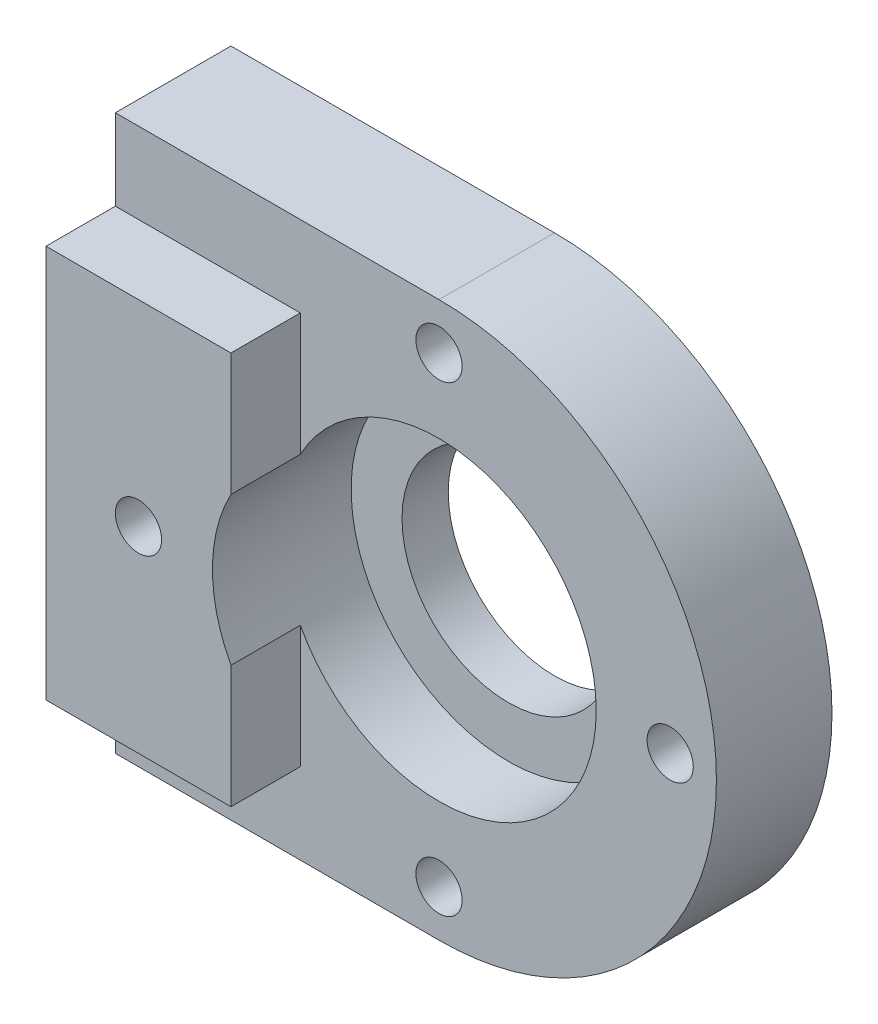
ISO-10303-21;
HEADER;
FILE_DESCRIPTION(('STEP AP214'),'2;1');
FILE_NAME('part.step','',(''),(''),'','','');
FILE_SCHEMA(('AUTOMOTIVE_DESIGN { 1 0 10303 214 1 1 1 1 }'));
ENDSEC;
DATA;
#1=APPLICATION_CONTEXT('core data for automotive mechanical design processes');
#2=APPLICATION_PROTOCOL_DEFINITION('international standard','automotive_design',2000,#1);
#3=PRODUCT_CONTEXT('',#1,'mechanical');
#4=PRODUCT('Part','Part','',(#3));
#5=PRODUCT_RELATED_PRODUCT_CATEGORY('part','',(#4));
#6=PRODUCT_DEFINITION_FORMATION('','',#4);
#7=PRODUCT_DEFINITION_CONTEXT('part definition',#1,'design');
#8=PRODUCT_DEFINITION('design','',#6,#7);
#9=PRODUCT_DEFINITION_SHAPE('','',#8);
#10=(LENGTH_UNIT() NAMED_UNIT(*) SI_UNIT(.MILLI.,.METRE.));
#11=(NAMED_UNIT(*) PLANE_ANGLE_UNIT() SI_UNIT($,.RADIAN.));
#12=(NAMED_UNIT(*) SI_UNIT($,.STERADIAN.) SOLID_ANGLE_UNIT());
#13=UNCERTAINTY_MEASURE_WITH_UNIT(LENGTH_MEASURE(1.E-05),#10,'distance_accuracy_value','');
#14=(GEOMETRIC_REPRESENTATION_CONTEXT(3) GLOBAL_UNCERTAINTY_ASSIGNED_CONTEXT((#13)) GLOBAL_UNIT_ASSIGNED_CONTEXT((#10,
#11,#12)) REPRESENTATION_CONTEXT('',''));
#15=CARTESIAN_POINT('',(0.,0.,0.));
#16=DIRECTION('',(0.,0.,1.));
#17=DIRECTION('',(1.,0.,0.));
#18=AXIS2_PLACEMENT_3D('',#15,#16,#17);
#19=CARTESIAN_POINT('',(40.,102.5,40.));
#20=DIRECTION('',(-1.,0.,0.));
#21=DIRECTION('',(0.,0.,1.));
#22=AXIS2_PLACEMENT_3D('',#19,#20,#21);
#23=PLANE('',#22);
#24=DIRECTION('',(0.,1.,0.));
#25=VECTOR('',#24,1.);
#26=CARTESIAN_POINT('',(40.,102.5,25.));
#27=LINE('',#26,#25);
#28=CARTESIAN_POINT('',(40.,17.5,25.));
#29=VERTEX_POINT('',#28);
#30=CARTESIAN_POINT('',(40.,44.,25.));
#31=VERTEX_POINT('',#30);
#32=EDGE_CURVE('E142',#29,#31,#27,.T.);
#33=ORIENTED_EDGE('',*,*,#32,.T.);
#34=DIRECTION('',(0.,0.,1.));
#35=VECTOR('',#34,1.);
#36=CARTESIAN_POINT('',(40.,44.,25.));
#37=LINE('',#36,#35);
#38=CARTESIAN_POINT('',(40.,44.,40.));
#39=VERTEX_POINT('',#38);
#40=EDGE_CURVE('E126',#31,#39,#37,.T.);
#41=ORIENTED_EDGE('',*,*,#40,.T.);
#42=DIRECTION('',(0.,1.,0.));
#43=VECTOR('',#42,1.);
#44=CARTESIAN_POINT('',(40.,102.5,40.));
#45=LINE('',#44,#43);
#46=CARTESIAN_POINT('',(40.,17.5,40.));
#47=VERTEX_POINT('',#46);
#48=EDGE_CURVE('E212',#47,#39,#45,.T.);
#49=ORIENTED_EDGE('',*,*,#48,.F.);
#50=DIRECTION('',(0.,0.,-1.));
#51=VECTOR('',#50,1.);
#52=CARTESIAN_POINT('',(40.,17.5,40.));
#53=LINE('',#52,#51);
#54=EDGE_CURVE('E153',#47,#29,#53,.T.);
#55=ORIENTED_EDGE('',*,*,#54,.T.);
#56=EDGE_LOOP('',(#33,#41,#49,#55));
#57=FACE_BOUND('',#56,.T.);
#58=ADVANCED_FACE('F44',(#57),#23,.F.);
#59=CARTESIAN_POINT('',(0.,120.,25.));
#60=DIRECTION('',(1.,0.,0.));
#61=DIRECTION('',(0.,0.,-1.));
#62=AXIS2_PLACEMENT_3D('',#59,#60,#61);
#63=PLANE('',#62);
#64=DIRECTION('',(0.,-1.,0.));
#65=VECTOR('',#64,1.);
#66=CARTESIAN_POINT('',(0.,120.,0.));
#67=LINE('',#66,#65);
#68=CARTESIAN_POINT('',(0.,120.,0.));
#69=VERTEX_POINT('',#68);
#70=CARTESIAN_POINT('',(0.,0.,0.));
#71=VERTEX_POINT('',#70);
#72=EDGE_CURVE('E158',#69,#71,#67,.T.);
#73=ORIENTED_EDGE('',*,*,#72,.T.);
#74=DIRECTION('',(0.,0.,-1.));
#75=VECTOR('',#74,1.);
#76=CARTESIAN_POINT('',(0.,0.,25.));
#77=LINE('',#76,#75);
#78=CARTESIAN_POINT('',(0.,0.,25.));
#79=VERTEX_POINT('',#78);
#80=EDGE_CURVE('E11',#79,#71,#77,.T.);
#81=ORIENTED_EDGE('',*,*,#80,.F.);
#82=DIRECTION('',(0.,-1.,0.));
#83=VECTOR('',#82,1.);
#84=CARTESIAN_POINT('',(0.,120.,25.));
#85=LINE('',#84,#83);
#86=CARTESIAN_POINT('',(0.,17.5,25.));
#87=VERTEX_POINT('',#86);
#88=EDGE_CURVE('E165',#87,#79,#85,.T.);
#89=ORIENTED_EDGE('',*,*,#88,.F.);
#90=DIRECTION('',(0.,0.,-1.));
#91=VECTOR('',#90,1.);
#92=CARTESIAN_POINT('',(0.,17.5,40.));
#93=LINE('',#92,#91);
#94=CARTESIAN_POINT('',(0.,17.5,40.));
#95=VERTEX_POINT('',#94);
#96=EDGE_CURVE('E159',#95,#87,#93,.T.);
#97=ORIENTED_EDGE('',*,*,#96,.F.);
#98=DIRECTION('',(0.,-1.,0.));
#99=VECTOR('',#98,1.);
#100=CARTESIAN_POINT('',(0.,17.5,40.));
#101=LINE('',#100,#99);
#102=CARTESIAN_POINT('',(0.,102.5,40.));
#103=VERTEX_POINT('',#102);
#104=EDGE_CURVE('E150',#103,#95,#101,.T.);
#105=ORIENTED_EDGE('',*,*,#104,.F.);
#106=DIRECTION('',(0.,0.,-1.));
#107=VECTOR('',#106,1.);
#108=CARTESIAN_POINT('',(0.,102.5,40.));
#109=LINE('',#108,#107);
#110=CARTESIAN_POINT('',(0.,102.5,25.));
#111=VERTEX_POINT('',#110);
#112=EDGE_CURVE('E149',#103,#111,#109,.T.);
#113=ORIENTED_EDGE('',*,*,#112,.T.);
#114=CARTESIAN_POINT('',(0.,120.,25.));
#115=VERTEX_POINT('',#114);
#116=EDGE_CURVE('E163',#115,#111,#85,.T.);
#117=ORIENTED_EDGE('',*,*,#116,.F.);
#118=DIRECTION('',(0.,0.,-1.));
#119=VECTOR('',#118,1.);
#120=CARTESIAN_POINT('',(0.,120.,25.));
#121=LINE('',#120,#119);
#122=EDGE_CURVE('E167',#115,#69,#121,.T.);
#123=ORIENTED_EDGE('',*,*,#122,.T.);
#124=EDGE_LOOP('',(#73,#81,#89,#97,#105,#113,#117,#123));
#125=FACE_BOUND('',#124,.T.);
#126=ADVANCED_FACE('F50',(#125),#63,.F.);
#127=CARTESIAN_POINT('',(0.,0.,25.));
#128=DIRECTION('',(0.,1.,0.));
#129=DIRECTION('',(0.,0.,1.));
#130=AXIS2_PLACEMENT_3D('',#127,#128,#129);
#131=PLANE('',#130);
#132=DIRECTION('',(1.,0.,0.));
#133=VECTOR('',#132,1.);
#134=CARTESIAN_POINT('',(0.,0.,0.));
#135=LINE('',#134,#133);
#136=CARTESIAN_POINT('',(70.,0.,0.));
#137=VERTEX_POINT('',#136);
#138=EDGE_CURVE('E173',#71,#137,#135,.T.);
#139=ORIENTED_EDGE('',*,*,#138,.T.);
#140=DIRECTION('',(0.,0.,-1.));
#141=VECTOR('',#140,1.);
#142=CARTESIAN_POINT('',(70.,0.,25.));
#143=LINE('',#142,#141);
#144=CARTESIAN_POINT('',(70.,0.,25.));
#145=VERTEX_POINT('',#144);
#146=EDGE_CURVE('E53',#145,#137,#143,.T.);
#147=ORIENTED_EDGE('',*,*,#146,.F.);
#148=DIRECTION('',(1.,0.,0.));
#149=VECTOR('',#148,1.);
#150=CARTESIAN_POINT('',(0.,0.,25.));
#151=LINE('',#150,#149);
#152=EDGE_CURVE('E161',#79,#145,#151,.T.);
#153=ORIENTED_EDGE('',*,*,#152,.F.);
#154=ORIENTED_EDGE('',*,*,#80,.T.);
#155=EDGE_LOOP('',(#139,#147,#153,#154));
#156=FACE_BOUND('',#155,.T.);
#157=ADVANCED_FACE('F288',(#156),#131,.F.);
#158=CARTESIAN_POINT('',(70.,60.,25.));
#159=DIRECTION('',(0.,0.,-1.));
#160=DIRECTION('',(-1.,0.,0.));
#161=AXIS2_PLACEMENT_3D('',#158,#159,#160);
#162=CYLINDRICAL_SURFACE('',#161,60.);
#163=CARTESIAN_POINT('',(70.,60.,0.));
#164=DIRECTION('',(0.,0.,1.));
#165=DIRECTION('',(1.,0.,0.));
#166=AXIS2_PLACEMENT_3D('',#163,#164,#165);
#167=CIRCLE('',#166,60.);
#168=CARTESIAN_POINT('',(70.,120.,0.));
#169=VERTEX_POINT('',#168);
#170=EDGE_CURVE('E174',#137,#169,#167,.T.);
#171=ORIENTED_EDGE('',*,*,#170,.T.);
#172=DIRECTION('',(0.,0.,-1.));
#173=VECTOR('',#172,1.);
#174=CARTESIAN_POINT('',(70.,120.,25.));
#175=LINE('',#174,#173);
#176=CARTESIAN_POINT('',(70.,120.,25.));
#177=VERTEX_POINT('',#176);
#178=EDGE_CURVE('E181',#177,#169,#175,.T.);
#179=ORIENTED_EDGE('',*,*,#178,.F.);
#180=CARTESIAN_POINT('',(70.,60.,25.));
#181=DIRECTION('',(0.,0.,1.));
#182=DIRECTION('',(1.,0.,0.));
#183=AXIS2_PLACEMENT_3D('',#180,#181,#182);
#184=CIRCLE('',#183,60.);
#185=EDGE_CURVE('E168',#145,#177,#184,.T.);
#186=ORIENTED_EDGE('',*,*,#185,.F.);
#187=ORIENTED_EDGE('',*,*,#146,.T.);
#188=EDGE_LOOP('',(#171,#179,#186,#187));
#189=FACE_BOUND('',#188,.T.);
#190=ADVANCED_FACE('F186',(#189),#162,.T.);
#191=CARTESIAN_POINT('',(70.,120.,25.));
#192=DIRECTION('',(0.,-1.,0.));
#193=DIRECTION('',(0.,0.,-1.));
#194=AXIS2_PLACEMENT_3D('',#191,#192,#193);
#195=PLANE('',#194);
#196=DIRECTION('',(-1.,0.,0.));
#197=VECTOR('',#196,1.);
#198=CARTESIAN_POINT('',(70.,120.,0.));
#199=LINE('',#198,#197);
#200=EDGE_CURVE('E180',#169,#69,#199,.T.);
#201=ORIENTED_EDGE('',*,*,#200,.T.);
#202=ORIENTED_EDGE('',*,*,#122,.F.);
#203=DIRECTION('',(-1.,0.,0.));
#204=VECTOR('',#203,1.);
#205=CARTESIAN_POINT('',(70.,120.,25.));
#206=LINE('',#205,#204);
#207=EDGE_CURVE('E166',#177,#115,#206,.T.);
#208=ORIENTED_EDGE('',*,*,#207,.F.);
#209=ORIENTED_EDGE('',*,*,#178,.T.);
#210=EDGE_LOOP('',(#201,#202,#208,#209));
#211=FACE_BOUND('',#210,.T.);
#212=ADVANCED_FACE('F198',(#211),#195,.F.);
#213=CARTESIAN_POINT('',(70.,60.,25.));
#214=DIRECTION('',(0.,0.,1.));
#215=DIRECTION('',(1.,0.,0.));
#216=AXIS2_PLACEMENT_3D('',#213,#214,#215);
#217=PLANE('',#216);
#218=CARTESIAN_POINT('',(70.,110.,25.));
#219=DIRECTION('',(0.,0.,1.));
#220=DIRECTION('',(1.,0.,0.));
#221=AXIS2_PLACEMENT_3D('',#218,#219,#220);
#222=CIRCLE('',#221,4.99999999999999);
#223=CARTESIAN_POINT('',(75.,110.,25.));
#224=VERTEX_POINT('',#223);
#225=EDGE_CURVE('E244',#224,#224,#222,.T.);
#226=ORIENTED_EDGE('',*,*,#225,.F.);
#227=EDGE_LOOP('',(#226));
#228=FACE_BOUND('',#227,.T.);
#229=CARTESIAN_POINT('',(120.,60.,25.));
#230=DIRECTION('',(0.,0.,1.));
#231=DIRECTION('',(1.,0.,0.));
#232=AXIS2_PLACEMENT_3D('',#229,#230,#231);
#233=CIRCLE('',#232,5.);
#234=CARTESIAN_POINT('',(125.,60.,25.));
#235=VERTEX_POINT('',#234);
#236=EDGE_CURVE('E237',#235,#235,#233,.T.);
#237=ORIENTED_EDGE('',*,*,#236,.F.);
#238=EDGE_LOOP('',(#237));
#239=FACE_BOUND('',#238,.T.);
#240=CARTESIAN_POINT('',(70.,10.,25.));
#241=DIRECTION('',(0.,0.,1.));
#242=DIRECTION('',(1.,0.,0.));
#243=AXIS2_PLACEMENT_3D('',#240,#241,#242);
#244=CIRCLE('',#243,5.);
#245=CARTESIAN_POINT('',(75.,10.,25.));
#246=VERTEX_POINT('',#245);
#247=EDGE_CURVE('E231',#246,#246,#244,.T.);
#248=ORIENTED_EDGE('',*,*,#247,.F.);
#249=EDGE_LOOP('',(#248));
#250=FACE_BOUND('',#249,.T.);
#251=CARTESIAN_POINT('',(70.,60.,25.));
#252=DIRECTION('',(0.,0.,1.));
#253=DIRECTION('',(1.,0.,0.));
#254=AXIS2_PLACEMENT_3D('',#251,#252,#253);
#255=CIRCLE('',#254,34.);
#256=CARTESIAN_POINT('',(40.,76.,25.));
#257=VERTEX_POINT('',#256);
#258=EDGE_CURVE('E129',#31,#257,#255,.T.);
#259=ORIENTED_EDGE('',*,*,#258,.F.);
#260=ORIENTED_EDGE('',*,*,#32,.F.);
#261=DIRECTION('',(1.,0.,0.));
#262=VECTOR('',#261,1.);
#263=CARTESIAN_POINT('',(40.,17.5,25.));
#264=LINE('',#263,#262);
#265=EDGE_CURVE('E68',#87,#29,#264,.T.);
#266=ORIENTED_EDGE('',*,*,#265,.F.);
#267=ORIENTED_EDGE('',*,*,#88,.T.);
#268=ORIENTED_EDGE('',*,*,#152,.T.);
#269=ORIENTED_EDGE('',*,*,#185,.T.);
#270=ORIENTED_EDGE('',*,*,#207,.T.);
#271=ORIENTED_EDGE('',*,*,#116,.T.);
#272=DIRECTION('',(-1.,0.,0.));
#273=VECTOR('',#272,1.);
#274=CARTESIAN_POINT('',(0.,102.5,25.));
#275=LINE('',#274,#273);
#276=CARTESIAN_POINT('',(40.,102.5,25.));
#277=VERTEX_POINT('',#276);
#278=EDGE_CURVE('E136',#277,#111,#275,.T.);
#279=ORIENTED_EDGE('',*,*,#278,.F.);
#280=EDGE_CURVE('E62',#257,#277,#27,.T.);
#281=ORIENTED_EDGE('',*,*,#280,.F.);
#282=EDGE_LOOP('',(#259,#260,#266,#267,#268,#269,#270,#271,#279,#281));
#283=FACE_BOUND('',#282,.T.);
#284=ADVANCED_FACE('F139',(#228,#239,#250,#283),#217,.T.);
#285=CARTESIAN_POINT('',(70.,60.,0.));
#286=DIRECTION('',(0.,0.,1.));
#287=DIRECTION('',(1.,0.,0.));
#288=AXIS2_PLACEMENT_3D('',#285,#286,#287);
#289=PLANE('',#288);
#290=CARTESIAN_POINT('',(70.,110.,0.));
#291=DIRECTION('',(0.,0.,1.));
#292=DIRECTION('',(1.,0.,0.));
#293=AXIS2_PLACEMENT_3D('',#290,#291,#292);
#294=CIRCLE('',#293,4.99999999999999);
#295=CARTESIAN_POINT('',(75.,110.,0.));
#296=VERTEX_POINT('',#295);
#297=EDGE_CURVE('E229',#296,#296,#294,.T.);
#298=ORIENTED_EDGE('',*,*,#297,.T.);
#299=EDGE_LOOP('',(#298));
#300=FACE_BOUND('',#299,.T.);
#301=CARTESIAN_POINT('',(120.,60.,0.));
#302=DIRECTION('',(0.,0.,1.));
#303=DIRECTION('',(1.,0.,0.));
#304=AXIS2_PLACEMENT_3D('',#301,#302,#303);
#305=CIRCLE('',#304,5.);
#306=CARTESIAN_POINT('',(125.,60.,0.));
#307=VERTEX_POINT('',#306);
#308=EDGE_CURVE('E245',#307,#307,#305,.T.);
#309=ORIENTED_EDGE('',*,*,#308,.T.);
#310=EDGE_LOOP('',(#309));
#311=FACE_BOUND('',#310,.T.);
#312=CARTESIAN_POINT('',(70.,10.,0.));
#313=DIRECTION('',(0.,0.,1.));
#314=DIRECTION('',(1.,0.,0.));
#315=AXIS2_PLACEMENT_3D('',#312,#313,#314);
#316=CIRCLE('',#315,5.);
#317=CARTESIAN_POINT('',(75.,10.,0.));
#318=VERTEX_POINT('',#317);
#319=EDGE_CURVE('E236',#318,#318,#316,.T.);
#320=ORIENTED_EDGE('',*,*,#319,.T.);
#321=EDGE_LOOP('',(#320));
#322=FACE_BOUND('',#321,.T.);
#323=CARTESIAN_POINT('',(70.,60.,0.));
#324=DIRECTION('',(0.,0.,1.));
#325=DIRECTION('',(1.,0.,0.));
#326=AXIS2_PLACEMENT_3D('',#323,#324,#325);
#327=CIRCLE('',#326,23.);
#328=CARTESIAN_POINT('',(93.,60.,0.));
#329=VERTEX_POINT('',#328);
#330=EDGE_CURVE('E47',#329,#329,#327,.T.);
#331=ORIENTED_EDGE('',*,*,#330,.T.);
#332=EDGE_LOOP('',(#331));
#333=FACE_BOUND('',#332,.T.);
#334=ORIENTED_EDGE('',*,*,#72,.F.);
#335=ORIENTED_EDGE('',*,*,#200,.F.);
#336=ORIENTED_EDGE('',*,*,#170,.F.);
#337=ORIENTED_EDGE('',*,*,#138,.F.);
#338=EDGE_LOOP('',(#334,#335,#336,#337));
#339=FACE_BOUND('',#338,.T.);
#340=ADVANCED_FACE('F199',(#300,#311,#322,#333,#339),#289,.F.);
#341=CARTESIAN_POINT('',(40.,17.5,40.));
#342=DIRECTION('',(0.,1.,0.));
#343=DIRECTION('',(0.,0.,1.));
#344=AXIS2_PLACEMENT_3D('',#341,#342,#343);
#345=PLANE('',#344);
#346=ORIENTED_EDGE('',*,*,#265,.T.);
#347=ORIENTED_EDGE('',*,*,#54,.F.);
#348=DIRECTION('',(1.,0.,0.));
#349=VECTOR('',#348,1.);
#350=CARTESIAN_POINT('',(40.,17.5,40.));
#351=LINE('',#350,#349);
#352=EDGE_CURVE('E213',#95,#47,#351,.T.);
#353=ORIENTED_EDGE('',*,*,#352,.F.);
#354=ORIENTED_EDGE('',*,*,#96,.T.);
#355=EDGE_LOOP('',(#346,#347,#353,#354));
#356=FACE_BOUND('',#355,.T.);
#357=ADVANCED_FACE('F291',(#356),#345,.F.);
#358=CARTESIAN_POINT('',(40.,76.,40.));
#359=VERTEX_POINT('',#358);
#360=CARTESIAN_POINT('',(40.,102.5,40.));
#361=VERTEX_POINT('',#360);
#362=EDGE_CURVE('E123',#359,#361,#45,.T.);
#363=ORIENTED_EDGE('',*,*,#362,.F.);
#364=DIRECTION('',(0.,0.,1.));
#365=VECTOR('',#364,1.);
#366=CARTESIAN_POINT('',(40.,76.,25.));
#367=LINE('',#366,#365);
#368=EDGE_CURVE('E125',#257,#359,#367,.T.);
#369=ORIENTED_EDGE('',*,*,#368,.F.);
#370=ORIENTED_EDGE('',*,*,#280,.T.);
#371=DIRECTION('',(0.,0.,-1.));
#372=VECTOR('',#371,1.);
#373=CARTESIAN_POINT('',(40.,102.5,40.));
#374=LINE('',#373,#372);
#375=EDGE_CURVE('E154',#361,#277,#374,.T.);
#376=ORIENTED_EDGE('',*,*,#375,.F.);
#377=EDGE_LOOP('',(#363,#369,#370,#376));
#378=FACE_BOUND('',#377,.T.);
#379=ADVANCED_FACE('F121',(#378),#23,.F.);
#380=CARTESIAN_POINT('',(0.,102.5,40.));
#381=DIRECTION('',(0.,-1.,0.));
#382=DIRECTION('',(0.,0.,-1.));
#383=AXIS2_PLACEMENT_3D('',#380,#381,#382);
#384=PLANE('',#383);
#385=ORIENTED_EDGE('',*,*,#278,.T.);
#386=ORIENTED_EDGE('',*,*,#112,.F.);
#387=DIRECTION('',(-1.,0.,0.));
#388=VECTOR('',#387,1.);
#389=CARTESIAN_POINT('',(0.,102.5,40.));
#390=LINE('',#389,#388);
#391=EDGE_CURVE('E151',#361,#103,#390,.T.);
#392=ORIENTED_EDGE('',*,*,#391,.F.);
#393=ORIENTED_EDGE('',*,*,#375,.T.);
#394=EDGE_LOOP('',(#385,#386,#392,#393));
#395=FACE_BOUND('',#394,.T.);
#396=ADVANCED_FACE('F210',(#395),#384,.F.);
#397=CARTESIAN_POINT('',(0.,0.,40.));
#398=DIRECTION('',(0.,0.,-1.));
#399=DIRECTION('',(-1.,0.,0.));
#400=AXIS2_PLACEMENT_3D('',#397,#398,#399);
#401=PLANE('',#400);
#402=CARTESIAN_POINT('',(20.,60.,40.));
#403=DIRECTION('',(0.,0.,1.));
#404=DIRECTION('',(1.,0.,0.));
#405=AXIS2_PLACEMENT_3D('',#402,#403,#404);
#406=CIRCLE('',#405,5.);
#407=CARTESIAN_POINT('',(25.,60.,40.));
#408=VERTEX_POINT('',#407);
#409=EDGE_CURVE('E227',#408,#408,#406,.T.);
#410=ORIENTED_EDGE('',*,*,#409,.F.);
#411=EDGE_LOOP('',(#410));
#412=FACE_BOUND('',#411,.T.);
#413=ORIENTED_EDGE('',*,*,#48,.T.);
#414=CARTESIAN_POINT('',(70.,60.,40.));
#415=DIRECTION('',(0.,0.,1.));
#416=DIRECTION('',(1.,0.,0.));
#417=AXIS2_PLACEMENT_3D('',#414,#415,#416);
#418=CIRCLE('',#417,34.);
#419=EDGE_CURVE('E217',#359,#39,#418,.T.);
#420=ORIENTED_EDGE('',*,*,#419,.F.);
#421=ORIENTED_EDGE('',*,*,#362,.T.);
#422=ORIENTED_EDGE('',*,*,#391,.T.);
#423=ORIENTED_EDGE('',*,*,#104,.T.);
#424=ORIENTED_EDGE('',*,*,#352,.T.);
#425=EDGE_LOOP('',(#413,#420,#421,#422,#423,#424));
#426=FACE_BOUND('',#425,.T.);
#427=ADVANCED_FACE('F300',(#412,#426),#401,.F.);
#428=CARTESIAN_POINT('',(70.,60.,10.));
#429=DIRECTION('',(0.,0.,1.));
#430=DIRECTION('',(1.,0.,0.));
#431=AXIS2_PLACEMENT_3D('',#428,#429,#430);
#432=CYLINDRICAL_SURFACE('',#431,34.);
#433=CARTESIAN_POINT('',(70.,60.,10.));
#434=DIRECTION('',(0.,0.,1.));
#435=DIRECTION('',(1.,0.,0.));
#436=AXIS2_PLACEMENT_3D('',#433,#434,#435);
#437=CIRCLE('',#436,34.);
#438=CARTESIAN_POINT('',(104.,60.,10.));
#439=VERTEX_POINT('',#438);
#440=EDGE_CURVE('E132',#439,#439,#437,.T.);
#441=ORIENTED_EDGE('',*,*,#440,.F.);
#442=EDGE_LOOP('',(#441));
#443=FACE_BOUND('',#442,.T.);
#444=ORIENTED_EDGE('',*,*,#258,.T.);
#445=ORIENTED_EDGE('',*,*,#368,.T.);
#446=ORIENTED_EDGE('',*,*,#419,.T.);
#447=ORIENTED_EDGE('',*,*,#40,.F.);
#448=EDGE_LOOP('',(#444,#445,#446,#447));
#449=FACE_BOUND('',#448,.T.);
#450=ADVANCED_FACE('F131',(#443,#449),#432,.F.);
#451=CARTESIAN_POINT('',(70.,60.,10.));
#452=DIRECTION('',(0.,0.,1.));
#453=DIRECTION('',(1.,0.,0.));
#454=AXIS2_PLACEMENT_3D('',#451,#452,#453);
#455=PLANE('',#454);
#456=CARTESIAN_POINT('',(70.,60.,10.));
#457=DIRECTION('',(0.,0.,1.));
#458=DIRECTION('',(1.,0.,0.));
#459=AXIS2_PLACEMENT_3D('',#456,#457,#458);
#460=CIRCLE('',#459,23.);
#461=CARTESIAN_POINT('',(93.,60.,10.));
#462=VERTEX_POINT('',#461);
#463=EDGE_CURVE('E225',#462,#462,#460,.T.);
#464=ORIENTED_EDGE('',*,*,#463,.F.);
#465=EDGE_LOOP('',(#464));
#466=FACE_BOUND('',#465,.T.);
#467=ORIENTED_EDGE('',*,*,#440,.T.);
#468=EDGE_LOOP('',(#467));
#469=FACE_BOUND('',#468,.T.);
#470=ADVANCED_FACE('F324',(#466,#469),#455,.T.);
#471=CARTESIAN_POINT('',(70.,60.,-5.));
#472=DIRECTION('',(0.,0.,1.));
#473=DIRECTION('',(1.,0.,0.));
#474=AXIS2_PLACEMENT_3D('',#471,#472,#473);
#475=CYLINDRICAL_SURFACE('',#474,23.);
#476=ORIENTED_EDGE('',*,*,#463,.T.);
#477=EDGE_LOOP('',(#476));
#478=FACE_BOUND('',#477,.T.);
#479=ORIENTED_EDGE('',*,*,#330,.F.);
#480=EDGE_LOOP('',(#479));
#481=FACE_BOUND('',#480,.T.);
#482=ADVANCED_FACE('F327',(#478,#481),#475,.F.);
#483=CARTESIAN_POINT('',(20.,60.,25.));
#484=DIRECTION('',(0.,0.,1.));
#485=DIRECTION('',(1.,0.,0.));
#486=AXIS2_PLACEMENT_3D('',#483,#484,#485);
#487=CYLINDRICAL_SURFACE('',#486,5.);
#488=CARTESIAN_POINT('',(20.,60.,25.));
#489=DIRECTION('',(0.,0.,1.));
#490=DIRECTION('',(1.,0.,0.));
#491=AXIS2_PLACEMENT_3D('',#488,#489,#490);
#492=CIRCLE('',#491,5.);
#493=CARTESIAN_POINT('',(25.,60.,25.));
#494=VERTEX_POINT('',#493);
#495=EDGE_CURVE('E228',#494,#494,#492,.T.);
#496=ORIENTED_EDGE('',*,*,#495,.F.);
#497=EDGE_LOOP('',(#496));
#498=FACE_BOUND('',#497,.T.);
#499=ORIENTED_EDGE('',*,*,#409,.T.);
#500=EDGE_LOOP('',(#499));
#501=FACE_BOUND('',#500,.T.);
#502=ADVANCED_FACE('F279',(#498,#501),#487,.F.);
#503=CARTESIAN_POINT('',(20.,60.,25.));
#504=DIRECTION('',(0.,0.,1.));
#505=DIRECTION('',(1.,0.,0.));
#506=AXIS2_PLACEMENT_3D('',#503,#504,#505);
#507=PLANE('',#506);
#508=ORIENTED_EDGE('',*,*,#495,.T.);
#509=EDGE_LOOP('',(#508));
#510=FACE_BOUND('',#509,.T.);
#511=ADVANCED_FACE('F266',(#510),#507,.T.);
#512=CARTESIAN_POINT('',(70.,10.,0.));
#513=DIRECTION('',(0.,0.,1.));
#514=DIRECTION('',(1.,0.,0.));
#515=AXIS2_PLACEMENT_3D('',#512,#513,#514);
#516=CYLINDRICAL_SURFACE('',#515,5.);
#517=ORIENTED_EDGE('',*,*,#319,.F.);
#518=EDGE_LOOP('',(#517));
#519=FACE_BOUND('',#518,.T.);
#520=ORIENTED_EDGE('',*,*,#247,.T.);
#521=EDGE_LOOP('',(#520));
#522=FACE_BOUND('',#521,.T.);
#523=ADVANCED_FACE('F269',(#519,#522),#516,.F.);
#524=CARTESIAN_POINT('',(120.,60.,0.));
#525=DIRECTION('',(0.,0.,1.));
#526=DIRECTION('',(1.,0.,0.));
#527=AXIS2_PLACEMENT_3D('',#524,#525,#526);
#528=CYLINDRICAL_SURFACE('',#527,5.);
#529=ORIENTED_EDGE('',*,*,#308,.F.);
#530=EDGE_LOOP('',(#529));
#531=FACE_BOUND('',#530,.T.);
#532=ORIENTED_EDGE('',*,*,#236,.T.);
#533=EDGE_LOOP('',(#532));
#534=FACE_BOUND('',#533,.T.);
#535=ADVANCED_FACE('F257',(#531,#534),#528,.F.);
#536=CARTESIAN_POINT('',(70.,110.,0.));
#537=DIRECTION('',(0.,0.,1.));
#538=DIRECTION('',(1.,0.,0.));
#539=AXIS2_PLACEMENT_3D('',#536,#537,#538);
#540=CYLINDRICAL_SURFACE('',#539,4.99999999999999);
#541=ORIENTED_EDGE('',*,*,#297,.F.);
#542=EDGE_LOOP('',(#541));
#543=FACE_BOUND('',#542,.T.);
#544=ORIENTED_EDGE('',*,*,#225,.T.);
#545=EDGE_LOOP('',(#544));
#546=FACE_BOUND('',#545,.T.);
#547=ADVANCED_FACE('F254',(#543,#546),#540,.F.);
#548=CLOSED_SHELL('',(#58,#126,#157,#190,#212,#284,#340,#357,#379,#396,#427,#450,#470,#482,#502,
#511,#523,#535,#547));
#549=MANIFOLD_SOLID_BREP('B2',#548);
#550=ADVANCED_BREP_SHAPE_REPRESENTATION('',(#18,#549),#14);
#551=SHAPE_DEFINITION_REPRESENTATION(#9,#550);
ENDSEC;
END-ISO-10303-21;
